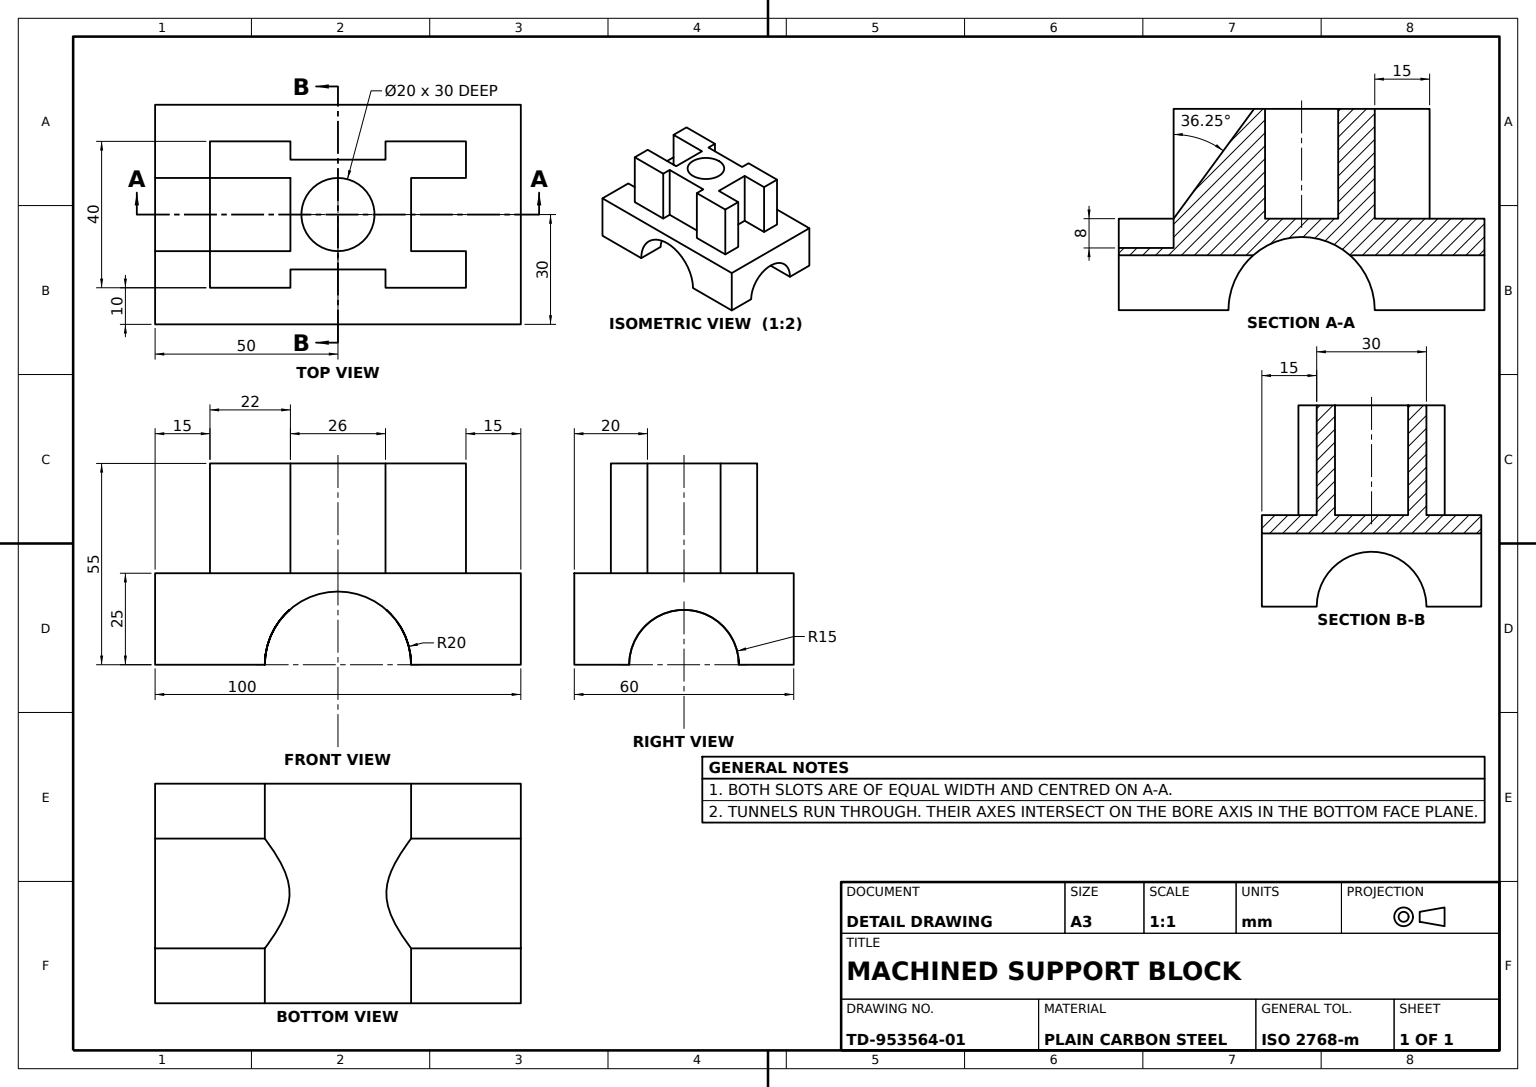
SolidWorks part; units mm, degrees
material "Plain Carbon Steel"
ref_plane "Front Plane" through (0, 0, 0) normal (0, 0, 1) x (1, 0, 0)
ref_plane "Top Plane" through (0, 0, 0) normal (0, 1, 0) x (1, 0, 0)
ref_plane "Right Plane" through (0, 0, 0) normal (1, 0, 0) x (0, 0, -1)
sketch "Base Arch Profile Sketch" plane through (0, 0, 0) normal (0, 0, 1) x (1, 0, 0)
  line L0 (20, -12.5) -> (50, -12.5)
  line L1 (-50, 12.5) -> (50, 12.5)
  line L2 (-50, 12.5) -> (-50, -12.5)
  line L3 (-50, -12.5) -> (-20, -12.5)
  line L4 (50, 12.5) -> (50, -12.5)
  line L5 (-50, 12.5) -> (50, -12.5) construction
  line L6 (-50, -12.5) -> (50, 12.5) construction
  arc A0 (20, -12.5) -> (-20, -12.5) centre (0, -12.5) ccw
  point P0 (0, 0)
  dimension "D1" = 100
  dimension "D3" = 20
  dimension "D4" = 30
  dimension "D2" = 25
extrude "Saddle Base Block" add sketch "Base Arch Profile Sketch" along normal mid plane 60
sketch "Through Hole Sketch" plane through (-50, 0, 0) normal (-1, 0, 0) x (0, 0, 1)
  line L0 (30, -12.5) -> (-30, -12.5) construction
  line L1 (-15, -12.5) -> (15, -12.5)
  arc A0 (15, -12.5) -> (-15, -12.5) centre (0, -12.5) ccw
  dimension "D1" = 15
extrude "Through Hole Ø15" cut sketch "Through Hole Sketch" against normal through all
sketch "Slot Profile Sketch" plane through (-50, 0, 0) normal (-1, 0, 0) x (0, 0, 1)
  line L0 (0, 12.5) -> (10, 12.5)
  line L1 (30, 12.5) -> (-30, 12.5) construction
  line L2 (10, 12.5) -> (10, 4.5)
  line L3 (10, 4.5) -> (-10, 4.5)
  line L4 (-10, 4.5) -> (-10, 12.5)
  line L5 (-10, 12.5) -> (0, 12.5)
  dimension "D1" = 20
  dimension "D2" = 8
  dimension "D3" = 10
extrude "Slot Cut" cut sketch "Slot Profile Sketch" against normal blind 15
sketch "Cross Boss Profile Sketch" plane through (0, 12.5, 0) normal (0, 1, 0) x (1, 0, 0)
  line L0 (0, 0) -> (20, 0) construction
  line L1 (35, 10) -> (35, 20) construction
  line L2 (50, 30) -> (-50, 30) construction
  line L3 (0, 0) -> (0, 30) construction
  line L5 (20, -10) -> (20, 10)
  line L6 (20, 10) -> (35, 10)
  line L7 (35, 10) -> (35, 20)
  line L8 (35, 20) -> (13, 20)
  line L9 (13, 20) -> (13, 15)
  line L10 (13, 15) -> (-13, 15)
  line L11 (-13, 15) -> (-13, 20)
  line L12 (-13, 20) -> (-35, 20)
  line L13 (-35, 20) -> (-35, 10)
  line L14 (-35, 10) -> (-20, 10)
  line L15 (-20, 10) -> (-20, -10)
  line L16 (20, -10) -> (35, -10)
  line L17 (35, -10) -> (35, -20)
  line L18 (35, -20) -> (13, -20)
  line L19 (13, -20) -> (13, -15)
  line L20 (-35, -10) -> (-20, -10)
  line L21 (-35, -20) -> (-35, -10)
  line L22 (-13, -15) -> (-13, -20)
  line L23 (-13, -20) -> (-35, -20)
  line L24 (13, -15) -> (-13, -15)
  circle A0 centre (0, 0) radius 10
  point P27 (-20, 0)
  dimension "D1" = 26
  dimension "D4" = 20
  dimension "D2" = 10
  dimension "D3" = 40
  dimension "D5" = 15
  dimension "D6" = 22
  dimension "D7" = 20
  dimension "D8" = 20
  dimension "D9" = 30
  dimension "D10" = 20
extrude "Cross Boss" add sketch "Cross Boss Profile Sketch" along normal blind 30
sketch "Upper Pad Sketch" plane through (-20, 0, 0) normal (-1, 0, 0) x (0, 0, 1)
  line L0 (-10, 42.5) -> (10, 42.5)
  line L1 (10, 42.5) -> (10, 12.5)
  line L2 (10, 12.5) -> (-10, 12.5)
  line L3 (-10, 12.5) -> (-10, 42.5)
extrude "Upper Pad" add sketch "Upper Pad Sketch" along normal blind 15
sketch "Notch Cut Sketch" plane through (0, 0, 20) normal (0, 0, 1) x (1, 0, 0)
  line L0 (-35, 12.5) -> (-13, 42.5)
  line L2 (-13, 42.5) -> (-35, 42.5)
  line L3 (-35, 42.5) -> (-35, 12.5)
extrude "Notch Cut" cut sketch "Notch Cut Sketch" against normal blind 30
sketch "Notch Fill Sketch" plane through (0, 0, 20) normal (0, 0, 1) x (1, 0, 0)
  line L0 (-35, 12.5) -> (-35, 42.5)
  line L1 (-35, 42.5) -> (-13, 42.5)
  line L2 (-13, 42.5) -> (-35, 12.5)
extrude "Notch Fill Boss" add sketch "Notch Fill Sketch" against normal blind 10
